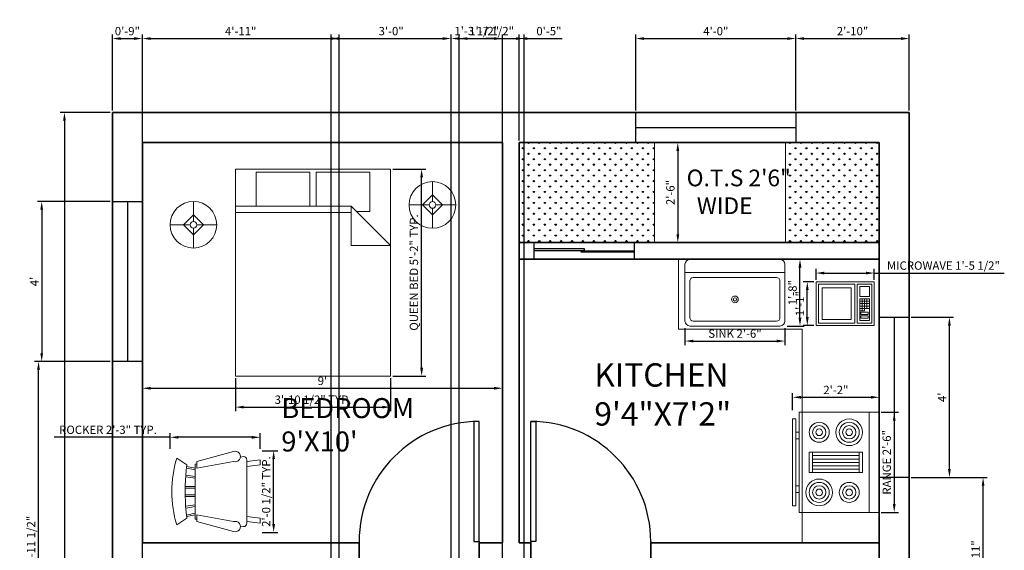
# Model space of a CAD drawing. Units: inches. Extents: x 2459 to 2755, y 1300 to 1776.
# Tile 4 of 4: x 2459 to 2755, y 1617 to 1776. Entities that reach past the tile are written whole.
import ezdxf

# ---------------------------------------------------------------- set-up
doc = ezdxf.new("R2010")
doc.units = ezdxf.units.IN
for name, color, linetype, lineweight in [('A-AREA-IDEN', 3, 'Continuous', 25), ('A-EQPM', 9, 'Continuous', 18), ('A-FLOR-CASE', 7, 'Continuous', 20), ('A-FLOR-FIXT', 8, 'Continuous', 18), ('A-WALL', 7, 'Continuous', 35), ('DIM', 4, 'Continuous', 18), ('DOOR', 20, 'Continuous', 25), ('FURNITURE', 6, 'Continuous', 18), ('L-PLNT', 3, 'Continuous', 18), ('L-PLNT-PATT', 8, 'Continuous', 13), ('WIN', 2, 'Continuous', 25)]:
    doc.layers.add(name, color=color, linetype=linetype, lineweight=lineweight)
doc.styles.get("Standard").update_dxf_attribs({"font": 'arial.ttf'})
doc.dimstyles.new('ISO-25', dxfattribs={"dimtxt": 2.5, "dimasz": 2.5, "dimexe": 1.25, "dimexo": 0.625, "dimtad": 1, "dimlunit": 3, "dimtxsty": 'Standard', "dimcen": 2.5, "dimadec": 0, "dimazin": 0, "dimtfac": 1, "dimtmove": 0, "dimatfit": 3, "dimfxl": 1, "dimarcsym": 0})

# ---------------------------------------------------------------- blocks, each defined once
blk = doc.blocks.new('*U2')
for p, q in [((0, 0), (0, -6)), ((40, 0), (40, -6))]:
    blk.add_line(p, q)
blk.add_lwpolyline([(0, 0), (0, 40), (1.75, 40), (1.75, 0)], close=True)
blk.add_arc((0, 0), 40, 0, 90)
blk = doc.blocks.new('*U3')
for p, q in [((0, 0), (0, -6)), ((-40, 0), (-40, -6))]:
    blk.add_line(p, q)
blk.add_lwpolyline([(0, 0), (0, 40), (-1.75, 40), (-1.75, 0)], close=True)
blk.add_arc((0, 0), 40, 90, 180)
blk = doc.blocks.new('Bed - Queen')
for p, q in [((0, -80.00003), (0, 0)), ((0, 0), (59.99999, 0)), ((59.99999, 0), (59.99999, -80.00003)), ((7.99999, -1.2), (28.79998, -1.2)), ((7.99999, -14.4), (7.99999, -1.2)), ((28.79998, -1.2), (28.79998, -14.4)), ((31.19999, -1.2), (51.99999, -1.2)), ((31.19999, -14.4), (31.19999, -1.2)), ((51.99999, -1.2), (51.99999, -16.4)), ((0, -14.4), (44.8, -14.4)), ((59.99999, -29.6), (44.8, -14.4)), ((44.8, -14.4), (44.8, -29.6)), ((44.8, -16.8), (0, -16.8)), ((51.99999, -16.4), (46.79936, -16.4)), ((44.8, -29.6), (59.99999, -29.6)), ((59.99999, -80.00003), (0, -80.00003))]:
    blk.add_line(p, q)
blk = doc.blocks.new('Microwave')
for p, q in [((18, 10), (22, 10)), ((22, 9), (18, 9)), ((19, 7), (19, 11)), ((20, 11), (20, 7)), ((21, 7), (21, 11)), ((18, 8), (22, 8)), ((22, 7), (18, 7)), ((20, 6), (18, 6)), ((19, 6), (19, 7)), ((20, 7), (20, 6))]:
    blk.add_line(p, q)
for points in [[(0, 0), (0, 18), (24, 18), (24, 0)], [(1, 1), (1, 17), (16, 17), (16, 1)], [(17, 1), (17, 17), (23, 17), (23, 1)], [(2.5, 2.5), (2.5, 15.5), (14.5, 15.5), (14.5, 2.5)], [(18, 12), (18, 16), (22, 16), (22, 12)], [(18, 2), (18, 11), (22, 11), (22, 2)], [(18.5, 4.5), (18.5, 5.5), (21.5, 5.5), (21.5, 4.5)], [(18.5, 3), (18.5, 4), (21.5, 4), (21.5, 3)]]:
    blk.add_lwpolyline(points, close=True)
blk = doc.blocks.new('Range-Oven - 30 in top')
for p, q in [((0, -3), (30, -3)), ((12, -6), (18, -6)), ((13, -20), (13, -6)), ((14, -6), (14, -20)), ((15, -20), (15, -6)), ((16, -6), (16, -20)), ((17, -20), (17, -6)), ((18, -20), (12, -20)), ((6, -24), (6, -25)), ((8, -25), (8, -24)), ((22, -25), (22, -24)), ((24, -24), (24, -25))]:
    blk.add_line(p, q)
for points in [[(0, -24), (0, 0), (30, 0), (30, -24)], [(12, -21), (12, -5), (18, -5), (18, -21)], [(2, -26), (2, -25), (28, -25), (28, -26)]]:
    blk.add_lwpolyline(points, close=True)
for centre, radius in [((6, -9), 4), ((6, -9), 3), ((6, -9), 2), ((6, -9), 1), ((24, -9), 3), ((24, -9), 2), ((24, -9), 1), ((24, -18), 4), ((6, -18), 3), ((6, -18), 2), ((6, -18), 1), ((24, -18), 3), ((24, -18), 2), ((24, -18), 1)]:
    blk.add_circle(centre, radius)
blk = doc.blocks.new('Sink-single - 30 in top')
blk.add_line((-15, -3.999996), (15, -3.999996))
for points in [[(-13.5, 0), (13.5, 0)], [(-15, -18.499996), (-15, -1.5)], [(15, -1.5), (15, -18.499996)], [(-12.5, -5.499996), (12.5, -5.499996)], [(-13.5, -17.499996), (-13.5, -6.499996)], [(13.5, -6.499996), (13.5, -17.499996)], [(13.5, -19.999996), (-13.5, -19.999996)], [(12.5, -18.499996), (-12.5, -18.499996)]]:
    blk.add_lwpolyline(points)
for radius in [1, 0.5]:
    blk.add_circle((0, -11.999996), radius)
for centre, radius, start, end in [((-13.5, -1.5), 1.5, 90, 180), ((13.5, -1.5), 1.5, 0, 90), ((-12.5, -6.499996), 1, 90, 180), ((12.5, -6.499996), 1, 0, 90), ((-12.5, -17.499996), 1, 180, 270), ((12.5, -17.499996), 1, 270, 0), ((-13.5, -18.499996), 1.5, 180, 270), ((13.5, -18.499996), 1.5, 270, 0)]:
    blk.add_arc(centre, radius, start, end)
blk = doc.blocks.new('Lamp - Table')
for p, q in [((0, 7), (0, 1)), ((0, 3), (-3, 0)), ((3, 0), (0, 3)), ((-1, 0), (-7, 0)), ((-3, 0), (0, -3)), ((0, -3), (3, 0)), ((1, 0), (7, 0)), ((0, -1), (0, -7))]:
    blk.add_line(p, q)
for radius in [7, 1]:
    blk.add_circle((0, 0), radius)
blk = doc.blocks.new('Chair - Rocking')
for p, q in [((-8, -4.5), (-10, -1.5)), ((8, -4.5), (10, -1.5)), ((-7.5, -4.5), (-7, -7)), ((-6.5, -7), (-7.02225, -4.43)), ((-4.5, -7), (-4.96674, -4.19951)), ((-4, -7), (-4.40532, -4.16272)), ((-1.5, -4.05012), (-1.5, -7)), ((-1, -7), (-1, -4.05012)), ((1, -7), (1, -4.04655)), ((1.5, -4.05012), (1.5, -7)), ((4, -7), (4.40187, -4.18694)), ((4.5, -7), (4.96761, -4.19437)), ((6.5, -7), (7, -4.4057)), ((7.5, -4.5), (7, -7)), ((-9, -7.5), (-12, -18.49999)), ((-7, -7.5), (-9, -7.5)), ((-9, -18.49999), (-7, -7.5)), ((-8.23428, -6.99939), (-8.3093, -7.47958)), ((-8.23041, -7), (8.23915, -7)), ((7, -7.5), (9, -7.5)), ((9, -18.49999), (7, -7.5)), ((8.31071, -7.48854), (8.23449, -7.00073)), ((9, -7.5), (12, -18.49999)), ((-10.36644, -20.64523), (-10.5, -21.49999)), ((10.5, -21.49999), (10.3575, -20.58798)), ((-9, -22.49999), (-9.5, -26.49999)), ((0, -22.49999), (-9.5, -22.49999)), ((-8, -26.49999), (-7.5, -22.49999)), ((0, -22.49999), (9.5, -22.49999)), ((8, -26.49999), (7.5, -22.49999)), ((9, -22.49999), (9.5, -26.49999)), ((-9.5, -26.49999), (-8, -26.49999)), ((9.5, -26.49999), (8, -26.49999))]:
    blk.add_line(p, q)
for centre, radius, start, end in [((0, -34.08333), 34.08333, 72.93847, 107.0615), ((0, -68.25004), 64.25, 93.92211, 97.15267), ((0, -68.25004), 64.25, 82.84733, 93.92211), ((-10.5, -18.99999), 1.58114, 161.5651, 18.43495), ((10.5, -18.99999), 1.58114, 161.5651, 18.43495), ((-9.5, -21.49999), 1, 180, 270), ((9.5, -21.49999), 1, 270, 0)]:
    blk.add_arc(centre, radius, start, end)
blk = doc.blocks.new('*D19')
at = {"layer": 'Defpoints', "color": 0, "transparency": 16777216}
for p in [(2487, 1748.32), (2472.62, 1324.32), (2487, 1324.32)]:
    blk.add_point(p, dxfattribs=at)
at = {"layer": 'DIM', "color": 0, "lineweight": -2, "transparency": 16777216}
for p, q in [((2486.37, 1748.32), (2471.37, 1748.32)), ((2472.62, 1745.82), (2472.62, 1326.82)), ((2486.37, 1324.32), (2471.37, 1324.32))]:
    blk.add_line(p, q, dxfattribs=at)
at = {"layer": 'DIM', "color": 0, "transparency": 16777216}
for points in [[(2472.2, 1745.82), (2473.04, 1745.82), (2472.62, 1748.32)], [(2472.2, 1326.82), (2473.04, 1326.82), (2472.62, 1324.32)]]:
    blk.add_solid(points, dxfattribs=at)
at = {"layer": 'DIM', "color": 0, "transparency": 16777216, "insert": (2470.72, 1536.32), "char_height": 2.5, "attachment_point": 5, "rotation": 90}
blk.add_mtext('35\'-4"', dxfattribs=at)
blk = doc.blocks.new('*D20')
at = {"layer": 'Defpoints', "color": 0, "transparency": 16777216}
for p in [(2487, 1721.67), (2465.8, 1673.67), (2487, 1673.67)]:
    blk.add_point(p, dxfattribs=at)
at = {"layer": 'DIM', "color": 0, "lineweight": -2, "transparency": 16777216}
for p, q in [((2486.37, 1721.67), (2464.55, 1721.67)), ((2465.8, 1719.17), (2465.8, 1676.17)), ((2486.37, 1673.67), (2464.55, 1673.67))]:
    blk.add_line(p, q, dxfattribs=at)
at = {"layer": 'DIM', "color": 0, "transparency": 16777216}
for points in [[(2465.38, 1719.17), (2466.22, 1719.17), (2465.8, 1721.67)], [(2465.38, 1676.17), (2466.22, 1676.17), (2465.8, 1673.67)]]:
    blk.add_solid(points, dxfattribs=at)
at = {"layer": 'DIM', "color": 0, "transparency": 16777216, "insert": (2463.93, 1697.67), "char_height": 2.5, "attachment_point": 5, "rotation": 90}
blk.add_mtext("4'", dxfattribs=at)
blk = doc.blocks.new('*D29')
at = {"layer": 'Defpoints', "color": 0, "transparency": 16777216}
for p in [(2726, 1686.95), (2738.05, 1686.95), (2726, 1638.95)]:
    blk.add_point(p, dxfattribs=at)
at = {"layer": 'DIM', "color": 0, "lineweight": -2, "transparency": 16777216}
for p, q in [((2726.62, 1686.95), (2739.3, 1686.95)), ((2738.05, 1641.45), (2738.05, 1684.45)), ((2726.62, 1638.95), (2739.3, 1638.95))]:
    blk.add_line(p, q, dxfattribs=at)
at = {"layer": 'DIM', "color": 0, "transparency": 16777216}
for points in [[(2737.63, 1684.45), (2738.46, 1684.45), (2738.05, 1686.95)], [(2737.63, 1641.45), (2738.46, 1641.45), (2738.05, 1638.95)]]:
    blk.add_solid(points, dxfattribs=at)
at = {"layer": 'DIM', "color": 0, "transparency": 16777216, "insert": (2736.17, 1662.95), "char_height": 2.5, "attachment_point": 5, "rotation": 90}
blk.add_mtext("4'", dxfattribs=at)
blk = doc.blocks.new('*D30')
at = {"layer": 'Defpoints', "color": 0, "transparency": 16777216}
for p in [(2649.55, 1739.32), (2649.55, 1709.32), (2656.59, 1709.32)]:
    blk.add_point(p, dxfattribs=at)
at = {"layer": 'DIM', "color": 0, "lineweight": -2, "transparency": 16777216}
for p, q in [((2650.18, 1739.32), (2657.84, 1739.32)), ((2656.59, 1736.82), (2656.59, 1711.82)), ((2650.18, 1709.32), (2657.84, 1709.32))]:
    blk.add_line(p, q, dxfattribs=at)
at = {"layer": 'DIM', "color": 0, "transparency": 16777216}
for points in [[(2656.17, 1736.82), (2657.01, 1736.82), (2656.59, 1739.32)], [(2656.17, 1711.82), (2657.01, 1711.82), (2656.59, 1709.32)]]:
    blk.add_solid(points, dxfattribs=at)
at = {"layer": 'DIM', "color": 0, "transparency": 16777216, "insert": (2654.69, 1724.32), "char_height": 2.5, "attachment_point": 5, "rotation": 90}
blk.add_mtext('2\'-6"', dxfattribs=at)
blk = doc.blocks.new('*D33')
at = {"layer": 'Defpoints', "color": 0, "transparency": 16777216}
for p in [(2496, 1665.67), (2604, 1665.67), (2604, 1665.67)]:
    blk.add_point(p, dxfattribs=at)
at = {"layer": 'DIM', "color": 0, "lineweight": -2, "transparency": 16777216}
for p, q in [((2496, 1666.29), (2496, 1666.92)), ((2498.5, 1665.67), (2601.5, 1665.67)), ((2604, 1666.29), (2604, 1666.92))]:
    blk.add_line(p, q, dxfattribs=at)
at = {"layer": 'DIM', "color": 0, "transparency": 16777216}
for points in [[(2498.5, 1666.09), (2498.5, 1665.25), (2496, 1665.67)], [(2601.5, 1666.09), (2601.5, 1665.25), (2604, 1665.67)]]:
    blk.add_solid(points, dxfattribs=at)
at = {"layer": 'DIM', "color": 0, "transparency": 16777216, "insert": (2550, 1667.57), "char_height": 2.5, "attachment_point": 5}
blk.add_mtext("9'", dxfattribs=at)
blk = doc.blocks.new('WIN-48IN')
blk.add_line((4.5, 48), (4.5, 0))
blk.add_lwpolyline([(0, 48), (9, 48), (9, 0), (0, 0)], close=True)
blk = doc.blocks.new('*D37')
at = {"layer": 'Defpoints', "color": 0, "transparency": 16777216}
for p in [(2570.45, 1731.37), (2579.75, 1731.37), (2570.45, 1669.32)]:
    blk.add_point(p, dxfattribs=at)
at = {"layer": 'DIM', "color": 0, "lineweight": -2, "transparency": 16777216}
for p, q in [((2571.07, 1731.37), (2581, 1731.37)), ((2579.75, 1671.82), (2579.75, 1728.87)), ((2571.07, 1669.32), (2581, 1669.32))]:
    blk.add_line(p, q, dxfattribs=at)
at = {"layer": 'DIM', "color": 0, "transparency": 16777216}
for points in [[(2579.34, 1728.87), (2580.17, 1728.87), (2579.75, 1731.37)], [(2579.34, 1671.82), (2580.17, 1671.82), (2579.75, 1669.32)]]:
    blk.add_solid(points, dxfattribs=at)
at = {"layer": 'DIM', "color": 0, "transparency": 16777216, "insert": (2577.76, 1700.35), "char_height": 2.5, "attachment_point": 5, "rotation": 90}
blk.add_mtext('QUEEN BED 5\'-2" TYP.', dxfattribs=at)
blk = doc.blocks.new('*D38')
at = {"layer": 'Defpoints', "color": 0, "transparency": 16777216}
for p in [(2523.91, 1669.32), (2570.45, 1669.32), (2570.45, 1660.02)]:
    blk.add_point(p, dxfattribs=at)
at = {"layer": 'DIM', "color": 0, "lineweight": -2, "transparency": 16777216}
for p, q in [((2523.91, 1668.7), (2523.91, 1658.77)), ((2570.45, 1668.7), (2570.45, 1658.77)), ((2526.41, 1660.02), (2567.95, 1660.02))]:
    blk.add_line(p, q, dxfattribs=at)
at = {"layer": 'DIM', "color": 0, "transparency": 16777216}
for points in [[(2526.41, 1660.43), (2526.41, 1659.6), (2523.91, 1660.02)], [(2567.95, 1660.43), (2567.95, 1659.6), (2570.45, 1660.02)]]:
    blk.add_solid(points, dxfattribs=at)
at = {"layer": 'DIM', "color": 0, "transparency": 16777216, "insert": (2547.18, 1661.93), "char_height": 2.5, "attachment_point": 5}
blk.add_mtext('3\'-10 1/2" TYP.', dxfattribs=at)
blk = doc.blocks.new('*D41')
at = {"layer": 'Defpoints', "color": 0, "transparency": 16777216}
for p in [(2504.32, 1650.98), (2504.32, 1646.93), (2531.32, 1646.93)]:
    blk.add_point(p, dxfattribs=at)
at = {"layer": 'DIM', "color": 0, "lineweight": -2, "transparency": 16777216}
for p, q in [((2504.32, 1650.98), (2469.55, 1650.98)), ((2504.32, 1647.55), (2504.32, 1652.23)), ((2528.82, 1650.98), (2506.82, 1650.98)), ((2531.32, 1647.55), (2531.32, 1652.23))]:
    blk.add_line(p, q, dxfattribs=at)
at = {"layer": 'DIM', "color": 0, "transparency": 16777216}
for points in [[(2506.82, 1651.39), (2506.82, 1650.56), (2504.32, 1650.98)], [(2528.82, 1651.39), (2528.82, 1650.56), (2531.32, 1650.98)]]:
    blk.add_solid(points, dxfattribs=at)
at = {"layer": 'DIM', "color": 0, "transparency": 16777216, "insert": (2485.68, 1652.9), "char_height": 2.5, "attachment_point": 5}
blk.add_mtext('ROCKER 2\'-3" TYP.', dxfattribs=at)
blk = doc.blocks.new('*D42')
at = {"layer": 'Defpoints', "color": 0, "transparency": 16777216}
for p in [(2531.32, 1646.93), (2535.37, 1646.93), (2531.32, 1622.49)]:
    blk.add_point(p, dxfattribs=at)
at = {"layer": 'DIM', "color": 0, "lineweight": -2, "transparency": 16777216}
for p, q in [((2531.94, 1646.93), (2536.62, 1646.93)), ((2535.37, 1624.99), (2535.37, 1644.43)), ((2531.94, 1622.49), (2536.62, 1622.49))]:
    blk.add_line(p, q, dxfattribs=at)
at = {"layer": 'DIM', "color": 0, "transparency": 16777216}
for points in [[(2534.95, 1644.43), (2535.79, 1644.43), (2535.37, 1646.93)], [(2534.95, 1624.99), (2535.79, 1624.99), (2535.37, 1622.49)]]:
    blk.add_solid(points, dxfattribs=at)
at = {"layer": 'DIM', "color": 0, "transparency": 16777216, "insert": (2533.45, 1634.71), "char_height": 2.5, "attachment_point": 5, "rotation": 90}
blk.add_mtext('2\'-0 1/2" TYP.', dxfattribs=at)
blk = doc.blocks.new('*D49')
at = {"layer": 'Defpoints', "color": 0, "transparency": 16777216}
for p in [(2715.51, 1700.19), (2698.05, 1697.57), (2715.51, 1697.57)]:
    blk.add_point(p, dxfattribs=at)
at = {"layer": 'DIM', "color": 0, "lineweight": -2, "transparency": 16777216}
for p, q in [((2698.05, 1698.2), (2698.05, 1701.44)), ((2715.51, 1698.2), (2715.51, 1701.44)), ((2700.55, 1700.19), (2713.01, 1700.19)), ((2715.51, 1700.19), (2754.51, 1700.19))]:
    blk.add_line(p, q, dxfattribs=at)
at = {"layer": 'DIM', "color": 0, "transparency": 16777216}
for points in [[(2700.55, 1700.61), (2700.55, 1699.78), (2698.05, 1700.19)], [(2713.01, 1700.61), (2713.01, 1699.78), (2715.51, 1700.19)]]:
    blk.add_solid(points, dxfattribs=at)
at = {"layer": 'DIM', "color": 0, "transparency": 16777216, "insert": (2736.26, 1702.11), "char_height": 2.5, "attachment_point": 5}
blk.add_mtext('MICROWAVE 1\'-5 1/2"', dxfattribs=at)
blk = doc.blocks.new('*D50')
at = {"layer": 'Defpoints', "color": 0, "transparency": 16777216}
for p in [(2695.43, 1697.57), (2698.05, 1697.57), (2698.05, 1684.48)]:
    blk.add_point(p, dxfattribs=at)
at = {"layer": 'DIM', "color": 0, "lineweight": -2, "transparency": 16777216}
for p, q in [((2697.42, 1697.57), (2694.18, 1697.57)), ((2695.43, 1686.98), (2695.43, 1695.07)), ((2697.42, 1684.48), (2694.18, 1684.48))]:
    blk.add_line(p, q, dxfattribs=at)
at = {"layer": 'DIM', "color": 0, "transparency": 16777216}
for points in [[(2695.01, 1695.07), (2695.84, 1695.07), (2695.43, 1697.57)], [(2695.01, 1686.98), (2695.84, 1686.98), (2695.43, 1684.48)]]:
    blk.add_solid(points, dxfattribs=at)
at = {"layer": 'DIM', "color": 0, "transparency": 16777216, "insert": (2693.55, 1691.02), "char_height": 2.5, "attachment_point": 5, "rotation": 90}
blk.add_mtext('1\'-1"', dxfattribs=at)
blk = doc.blocks.new('*D51')
at = {"layer": 'Defpoints', "color": 0, "transparency": 16777216}
for p in [(2717, 1658.47), (2717, 1628.47), (2721.5, 1628.47)]:
    blk.add_point(p, dxfattribs=at)
at = {"layer": 'DIM', "color": 0, "lineweight": -2, "transparency": 16777216}
for p, q in [((2717.62, 1658.47), (2722.75, 1658.47)), ((2721.5, 1655.97), (2721.5, 1630.97)), ((2717.62, 1628.47), (2722.75, 1628.47))]:
    blk.add_line(p, q, dxfattribs=at)
at = {"layer": 'DIM', "color": 0, "transparency": 16777216}
for points in [[(2721.08, 1655.97), (2721.91, 1655.97), (2721.5, 1658.47)], [(2721.08, 1630.97), (2721.91, 1630.97), (2721.5, 1628.47)]]:
    blk.add_solid(points, dxfattribs=at)
at = {"layer": 'DIM', "color": 0, "transparency": 16777216, "insert": (2719.58, 1643.47), "char_height": 2.5, "attachment_point": 5, "rotation": 90}
blk.add_mtext('RANGE 2\'-6"', dxfattribs=at)
blk = doc.blocks.new('*D52')
at = {"layer": 'Defpoints', "color": 0, "transparency": 16777216}
for p in [(2717, 1662.97), (2691, 1658.47), (2717, 1658.47)]:
    blk.add_point(p, dxfattribs=at)
at = {"layer": 'DIM', "color": 0, "lineweight": -2, "transparency": 16777216}
for p, q in [((2691, 1659.1), (2691, 1664.22)), ((2693.5, 1662.97), (2714.5, 1662.97)), ((2717, 1659.1), (2717, 1664.22))]:
    blk.add_line(p, q, dxfattribs=at)
at = {"layer": 'DIM', "color": 0, "transparency": 16777216}
for points in [[(2693.5, 1663.39), (2693.5, 1662.56), (2691, 1662.97)], [(2714.5, 1663.39), (2714.5, 1662.56), (2717, 1662.97)]]:
    blk.add_solid(points, dxfattribs=at)
at = {"layer": 'DIM', "color": 0, "transparency": 16777216, "insert": (2704, 1664.85), "char_height": 2.5, "attachment_point": 5}
blk.add_mtext('2\'-2"', dxfattribs=at)
blk = doc.blocks.new('*D53')
at = {"layer": 'Defpoints', "color": 0, "transparency": 16777216}
for p in [(2658.73, 1684.32), (2688.73, 1684.32), (2688.73, 1679.82)]:
    blk.add_point(p, dxfattribs=at)
at = {"layer": 'DIM', "color": 0, "lineweight": -2, "transparency": 16777216}
for p, q in [((2658.73, 1683.69), (2658.73, 1678.57)), ((2688.73, 1683.69), (2688.73, 1678.57)), ((2661.23, 1679.82), (2686.23, 1679.82))]:
    blk.add_line(p, q, dxfattribs=at)
at = {"layer": 'DIM', "color": 0, "transparency": 16777216}
for points in [[(2661.23, 1680.23), (2661.23, 1679.4), (2658.73, 1679.82)], [(2686.23, 1680.23), (2686.23, 1679.4), (2688.73, 1679.82)]]:
    blk.add_solid(points, dxfattribs=at)
at = {"layer": 'DIM', "color": 0, "transparency": 16777216, "insert": (2673.73, 1681.73), "char_height": 2.5, "attachment_point": 5}
blk.add_mtext('SINK 2\'-6"', dxfattribs=at)
blk = doc.blocks.new('*D54')
at = {"layer": 'Defpoints', "color": 0, "transparency": 16777216}
for p in [(2688.73, 1704.32), (2693.23, 1704.32), (2688.73, 1684.32)]:
    blk.add_point(p, dxfattribs=at)
at = {"layer": 'DIM', "color": 0, "lineweight": -2, "transparency": 16777216}
for p, q in [((2689.36, 1704.32), (2694.48, 1704.32)), ((2693.23, 1686.82), (2693.23, 1701.82)), ((2689.36, 1684.32), (2694.48, 1684.32))]:
    blk.add_line(p, q, dxfattribs=at)
at = {"layer": 'DIM', "color": 0, "transparency": 16777216}
for points in [[(2692.81, 1701.82), (2693.65, 1701.82), (2693.23, 1704.32)], [(2692.81, 1686.82), (2693.65, 1686.82), (2693.23, 1684.32)]]:
    blk.add_solid(points, dxfattribs=at)
at = {"layer": 'DIM', "color": 0, "transparency": 16777216, "insert": (2691.33, 1694.32), "char_height": 2.5, "attachment_point": 5, "rotation": 90}
blk.add_mtext('1\'-8"', dxfattribs=at)
blk = doc.blocks.new('*D58')
at = {"layer": 'Defpoints', "color": 0, "transparency": 16777216}
for p in [(2496, 1770.47), (2487, 1748.32), (2496, 1739.32)]:
    blk.add_point(p, dxfattribs=at)
at = {"layer": 'DIM', "color": 0, "lineweight": -2, "transparency": 16777216}
for p, q in [((2487, 1748.94), (2487, 1771.72)), ((2489.5, 1770.47), (2493.5, 1770.47)), ((2496, 1739.94), (2496, 1771.72))]:
    blk.add_line(p, q, dxfattribs=at)
at = {"layer": 'DIM', "color": 0, "transparency": 16777216}
for points in [[(2489.5, 1770.88), (2489.5, 1770.05), (2487, 1770.47)], [(2493.5, 1770.88), (2493.5, 1770.05), (2496, 1770.47)]]:
    blk.add_solid(points, dxfattribs=at)
at = {"layer": 'DIM', "color": 0, "transparency": 16777216, "insert": (2491.5, 1772.37), "char_height": 2.5, "attachment_point": 5}
blk.add_mtext('0\'-9"', dxfattribs=at)
blk = doc.blocks.new('*D59')
at = {"layer": 'Defpoints', "color": 0, "transparency": 16777216}
for p in [(2609, 1770.47), (2604, 1739.32), (2609, 1739.32)]:
    blk.add_point(p, dxfattribs=at)
at = {"layer": 'DIM', "color": 0, "lineweight": -2, "transparency": 16777216}
for p, q in [((2601.5, 1770.47), (2599, 1770.47)), ((2604, 1739.94), (2604, 1771.72)), ((2604, 1770.47), (2609, 1770.47)), ((2609, 1739.94), (2609, 1771.72)), ((2611.5, 1770.47), (2621.89, 1770.47))]:
    blk.add_line(p, q, dxfattribs=at)
at = {"layer": 'DIM', "color": 0, "transparency": 16777216}
for points in [[(2601.5, 1770.88), (2601.5, 1770.05), (2604, 1770.47)], [(2611.5, 1770.88), (2611.5, 1770.05), (2609, 1770.47)]]:
    blk.add_solid(points, dxfattribs=at)
at = {"layer": 'DIM', "color": 0, "transparency": 16777216, "insert": (2617.94, 1772.37), "char_height": 2.5, "attachment_point": 5}
blk.add_mtext('0\'-5"', dxfattribs=at)
blk = doc.blocks.new('*D60')
at = {"layer": 'Defpoints', "color": 0, "transparency": 16777216}
for p in [(2691.98, 1770.47), (2643.98, 1748.32), (2691.98, 1748.32)]:
    blk.add_point(p, dxfattribs=at)
at = {"layer": 'DIM', "color": 0, "lineweight": -2, "transparency": 16777216}
for p, q in [((2643.98, 1748.94), (2643.98, 1771.72)), ((2646.48, 1770.47), (2689.48, 1770.47)), ((2691.98, 1748.94), (2691.98, 1771.72))]:
    blk.add_line(p, q, dxfattribs=at)
at = {"layer": 'DIM', "color": 0, "transparency": 16777216}
for points in [[(2646.48, 1770.88), (2646.48, 1770.05), (2643.98, 1770.47)], [(2689.48, 1770.88), (2689.48, 1770.05), (2691.98, 1770.47)]]:
    blk.add_solid(points, dxfattribs=at)
at = {"layer": 'DIM', "color": 0, "transparency": 16777216, "insert": (2667.98, 1772.37), "char_height": 2.5, "attachment_point": 5}
blk.add_mtext('4\'-0"', dxfattribs=at)
blk = doc.blocks.new('*D61')
at = {"layer": 'Defpoints', "color": 0, "transparency": 16777216}
for p in [(2726, 1770.47), (2691.98, 1748.32), (2726, 1748.32)]:
    blk.add_point(p, dxfattribs=at)
at = {"layer": 'DIM', "color": 0, "lineweight": -2, "transparency": 16777216}
for p, q in [((2691.98, 1748.94), (2691.98, 1771.72)), ((2694.48, 1770.47), (2723.5, 1770.47)), ((2726, 1748.94), (2726, 1771.72))]:
    blk.add_line(p, q, dxfattribs=at)
at = {"layer": 'DIM', "color": 0, "transparency": 16777216}
for points in [[(2694.48, 1770.88), (2694.48, 1770.05), (2691.98, 1770.47)], [(2723.5, 1770.88), (2723.5, 1770.05), (2726, 1770.47)]]:
    blk.add_solid(points, dxfattribs=at)
at = {"layer": 'DIM', "color": 0, "transparency": 16777216, "insert": (2708.99, 1772.37), "char_height": 2.5, "attachment_point": 5}
blk.add_mtext('2\'-10"', dxfattribs=at)
blk = doc.blocks.new('*D64')
at = {"layer": 'Defpoints', "color": 0, "transparency": 16777216}
for p in [(2464.85, 1673.67), (2487, 1673.67), (2487, 1565.93)]:
    blk.add_point(p, dxfattribs=at)
at = {"layer": 'DIM', "color": 0, "lineweight": -2, "transparency": 16777216}
for p, q in [((2486.37, 1673.67), (2463.6, 1673.67)), ((2464.85, 1568.43), (2464.85, 1671.17)), ((2486.37, 1565.93), (2463.6, 1565.93))]:
    blk.add_line(p, q, dxfattribs=at)
at = {"layer": 'DIM', "color": 0, "transparency": 16777216}
for points in [[(2464.43, 1671.17), (2465.26, 1671.17), (2464.85, 1673.67)], [(2464.43, 1568.43), (2465.26, 1568.43), (2464.85, 1565.93)]]:
    blk.add_solid(points, dxfattribs=at)
at = {"layer": 'DIM', "color": 0, "transparency": 16777216, "insert": (2462.93, 1619.8), "char_height": 2.5, "attachment_point": 5, "rotation": 90}
blk.add_mtext('8\'-11 1/2"', dxfattribs=at)
blk = doc.blocks.new('*D69')
at = {"layer": 'Defpoints', "color": 0, "transparency": 16777216}
for p in [(2726, 1638.95), (2748.15, 1638.95), (2726, 1591.84)]:
    blk.add_point(p, dxfattribs=at)
at = {"layer": 'DIM', "color": 0, "lineweight": -2, "transparency": 16777216}
for p, q in [((2726.62, 1638.95), (2749.4, 1638.95)), ((2748.15, 1594.34), (2748.15, 1636.45)), ((2726.62, 1591.84), (2749.4, 1591.84))]:
    blk.add_line(p, q, dxfattribs=at)
at = {"layer": 'DIM', "color": 0, "transparency": 16777216}
for points in [[(2747.73, 1636.45), (2748.56, 1636.45), (2748.15, 1638.95)], [(2747.73, 1594.34), (2748.56, 1594.34), (2748.15, 1591.84)]]:
    blk.add_solid(points, dxfattribs=at)
at = {"layer": 'DIM', "color": 0, "transparency": 16777216, "insert": (2746.24, 1615.39), "char_height": 2.5, "attachment_point": 5, "rotation": 90}
blk.add_mtext('3\'-11"', dxfattribs=at)
blk = doc.blocks.new('*D70')
at = {"layer": 'Defpoints', "color": 0, "transparency": 16777216}
for p in [(2588.61, 1770.47), (2552.61, 1374.32), (2588.61, 1374.32)]:
    blk.add_point(p, dxfattribs=at)
at = {"layer": 'DIM', "color": 0, "lineweight": -2, "transparency": 16777216}
for p, q in [((2552.61, 1374.94), (2552.61, 1771.72)), ((2555.11, 1770.47), (2586.11, 1770.47)), ((2588.61, 1374.94), (2588.61, 1771.72))]:
    blk.add_line(p, q, dxfattribs=at)
at = {"layer": 'DIM', "color": 0, "transparency": 16777216}
for points in [[(2555.11, 1770.88), (2555.11, 1770.05), (2552.61, 1770.47)], [(2586.11, 1770.88), (2586.11, 1770.05), (2588.61, 1770.47)]]:
    blk.add_solid(points, dxfattribs=at)
at = {"layer": 'DIM', "color": 0, "transparency": 16777216, "insert": (2570.61, 1772.37), "char_height": 2.5, "attachment_point": 5}
blk.add_mtext('3\'-0"', dxfattribs=at)
blk = doc.blocks.new('*D77')
at = {"layer": 'Defpoints', "color": 0, "transparency": 16777216}
for p in [(2554.97, 1770.47), (2496, 1458.32), (2554.97, 1458.32)]:
    blk.add_point(p, dxfattribs=at)
at = {"layer": 'DIM', "color": 0, "lineweight": -2, "transparency": 16777216}
for p, q in [((2496, 1458.94), (2496, 1771.72)), ((2498.5, 1770.47), (2552.47, 1770.47)), ((2554.97, 1458.94), (2554.97, 1771.72))]:
    blk.add_line(p, q, dxfattribs=at)
at = {"layer": 'DIM', "color": 0, "transparency": 16777216}
for points in [[(2498.5, 1770.88), (2498.5, 1770.05), (2496, 1770.47)], [(2552.47, 1770.88), (2552.47, 1770.05), (2554.97, 1770.47)]]:
    blk.add_solid(points, dxfattribs=at)
at = {"layer": 'DIM', "color": 0, "transparency": 16777216, "insert": (2525.48, 1772.35), "char_height": 2.5, "attachment_point": 5}
blk.add_mtext('4\'-11"', dxfattribs=at)
blk = doc.blocks.new('*D78')
at = {"layer": 'Defpoints', "color": 0, "transparency": 16777216}
for p in [(2610.51, 1770.47), (2590.97, 1458.32), (2610.51, 1458.32)]:
    blk.add_point(p, dxfattribs=at)
at = {"layer": 'DIM', "color": 0, "lineweight": -2, "transparency": 16777216}
for p, q in [((2590.97, 1458.94), (2590.97, 1771.72)), ((2593.47, 1770.47), (2608.01, 1770.47)), ((2610.51, 1458.94), (2610.51, 1771.72))]:
    blk.add_line(p, q, dxfattribs=at)
at = {"layer": 'DIM', "color": 0, "transparency": 16777216}
for points in [[(2593.47, 1770.88), (2593.47, 1770.05), (2590.97, 1770.47)], [(2608.01, 1770.88), (2608.01, 1770.05), (2610.51, 1770.47)]]:
    blk.add_solid(points, dxfattribs=at)
at = {"layer": 'DIM', "color": 0, "transparency": 16777216, "insert": (2600.74, 1772.38), "char_height": 2.5, "attachment_point": 5}
blk.add_mtext('1\'-7 1/2"', dxfattribs=at)
blk = doc.blocks.new('*D79')
at = {"layer": 'Defpoints', "color": 0, "transparency": 16777216}
for p in [(2604, 1770.47), (2588.61, 1374.32), (2604, 1374.32)]:
    blk.add_point(p, dxfattribs=at)
at = {"layer": 'DIM', "color": 0, "lineweight": -2, "transparency": 16777216}
for p, q in [((2588.61, 1374.94), (2588.61, 1771.72)), ((2591.11, 1770.47), (2601.5, 1770.47)), ((2604, 1374.94), (2604, 1771.72))]:
    blk.add_line(p, q, dxfattribs=at)
at = {"layer": 'DIM', "color": 0, "transparency": 16777216}
for points in [[(2591.11, 1770.88), (2591.11, 1770.05), (2588.61, 1770.47)], [(2601.5, 1770.88), (2601.5, 1770.05), (2604, 1770.47)]]:
    blk.add_solid(points, dxfattribs=at)
at = {"layer": 'DIM', "color": 0, "transparency": 16777216, "insert": (2596.3, 1772.39), "char_height": 2.5, "attachment_point": 5}
blk.add_mtext('1\'-3 1/2"', dxfattribs=at)

msp = doc.modelspace()

# ---------------------------------------------------------------- hatches: boundary and pattern name
at = {"layer": 'L-PLNT-PATT', "transparency": 33554503}
h = msp.add_hatch(dxfattribs=at)
h.set_pattern_fill('GRASS', color=256, scale=0.091)
h.paths.add_polyline_path([(2649.551, 1739.317), (2608.997, 1739.317), (2608.997, 1709.317), (2649.551, 1709.317)])
h.paths.add_polyline_path([(2716.997, 1739.317), (2688.842, 1739.317), (2688.842, 1709.317), (2716.997, 1709.317)])

# ---------------------------------------------------------------- linework, layer by layer
at = {"layer": 'A-FLOR-CASE'}
for points in [[(2716.997, 1683.35), (2716.997, 1704.317), (2656.778, 1704.317), (2656.778, 1683.35), (2693.912, 1683.35)], [(2693.912, 1704.317), (2716.997, 1704.317), (2716.997, 1619.317), (2693.912, 1619.317), (2693.912, 1683.35)]]:
    msp.add_lwpolyline(points, dxfattribs=at)
at = {"layer": 'A-WALL'}
for p, q in [((2486.997, 1324.317), (2486.997, 1748.317)), ((2486.997, 1748.317), (2725.997, 1748.317)), ((2725.997, 1324.317), (2725.997, 1748.317)), ((2495.997, 1739.317), (2603.997, 1739.317)), ((2495.997, 1619.317), (2495.997, 1739.317)), ((2603.997, 1619.317), (2603.997, 1739.317)), ((2608.997, 1619.317), (2608.997, 1739.317)), ((2608.997, 1739.317), (2716.997, 1739.317)), ((2716.997, 1333.317), (2716.997, 1739.317)), ((2608.997, 1709.317), (2716.997, 1709.317)), ((2608.997, 1704.317), (2716.997, 1704.317)), ((2495.997, 1619.317), (2560.996, 1619.317)), ((2596.996, 1619.317), (2603.997, 1619.317)), ((2608.997, 1619.317), (2612.476, 1619.317)), ((2648.476, 1619.317), (2716.997, 1619.317))]:
    msp.add_line(p, q, dxfattribs=at)
for points in [[(2560.996, 1614.317), (2560.996, 1619.317)], [(2596.996, 1619.317), (2596.996, 1614.317)], [(2612.476, 1614.317), (2612.476, 1619.317)], [(2648.476, 1619.317), (2648.476, 1614.317)]]:
    msp.add_lwpolyline(points, dxfattribs=at)
at = {"layer": 'DOOR'}
for points in [[(2613.521, 1704.317), (2613.521, 1709.317), (2643.521, 1709.317), (2643.521, 1704.317)], [(2613.521, 1707.548), (2628.521, 1707.548), (2628.521, 1706.817), (2613.521, 1706.817)], [(2627.635, 1706.817), (2643.521, 1706.817), (2643.521, 1706.465), (2627.635, 1706.465)]]:
    msp.add_lwpolyline(points, close=True, dxfattribs=at)
at = {"layer": 'L-PLNT'}
for points in [[(2608.997, 1739.317), (2649.551, 1739.317), (2649.551, 1709.317), (2608.997, 1709.317)], [(2716.997, 1709.317), (2688.842, 1709.317), (2688.842, 1739.317), (2716.997, 1739.317)]]:
    msp.add_lwpolyline(points, close=True, dxfattribs=at)

# ---------------------------------------------------------------- block references
at = {"layer": 'A-EQPM', "xscale": 0.7276770498572076, "yscale": 0.7276770498572076, "zscale": 0.7276770498572076}
msp.add_blockref('Microwave', (2698.046, 1684.475), dxfattribs=at)
at = {"layer": 'A-EQPM', "rotation": 270}
msp.add_blockref('Range-Oven - 30 in top', (2716.997, 1658.474), dxfattribs=at)
at = {"layer": 'A-FLOR-FIXT'}
msp.add_blockref('Sink-single - 30 in top', (2673.731, 1704.317), dxfattribs=at)
at = {"layer": 'DOOR', "xscale": 0.9, "yscale": 0.9, "zscale": 0.9}
for name, p in [('*U3', (2596.996, 1619.717)), ('*U2', (2612.476, 1619.717))]:
    msp.add_blockref(name, p, dxfattribs=at)
at = {"layer": 'FURNITURE', "xscale": 0.775599459013597, "yscale": 0.775599459013597, "zscale": 0.775599459013597}
msp.add_blockref('Bed - Queen', (2523.911, 1731.371), dxfattribs=at)
at = {"layer": 'FURNITURE'}
for p in [(2582.994, 1720.599), (2511.315, 1714.666)]:
    msp.add_blockref('Lamp - Table', p, dxfattribs=at)
at = {"layer": 'FURNITURE', "rotation": 90}
msp.add_blockref('Chair - Rocking', (2504.82, 1634.71), dxfattribs=at)
at = {"layer": 'WIN', "rotation": 89.99999999999982}
msp.add_blockref('WIN-48IN', (2691.98, 1739.317), dxfattribs=at)
at = {"layer": 'WIN'}
for p in [(2486.997, 1673.674), (2716.997, 1638.951)]:
    msp.add_blockref('WIN-48IN', p, dxfattribs=at)

# ---------------------------------------------------------------- texts
at = {"layer": 'A-AREA-IDEN', "attachment_point": 1}
for s, insert, char_height in [('{O.T.S 2\'6"\\P  WIDE}', (2659.246, 1731.199), 5), ('{KITCHEN\\P9\'4"X7\'2"}', (2631.544, 1673.152), 7), ("{BEDROOM\\P9'X10'}", (2537.664, 1662.725), 6)]:
    msp.add_mtext_dynamic_manual_height_columns(s, width=133.04104, gutter_width=21.155, heights=[0], dxfattribs=dict(at, insert=insert, char_height=char_height))

# ---------------------------------------------------------------- dimensions: what is measured, and where the dimension line sits
at = {"layer": 'DIM'}
for base, p1, p2, override, picture, middle in [((2603.997, 1770.467), (2588.609, 1374.317), (2603.997, 1374.317), {"dimdec": 1, "dimlfac": 1, "dimrnd": 0, "dimzin": 1, "dimdsep": 46, "dimlunit": 4, "dimfrac": 2}, '*D79', (2596.303, 1772.386)), ((2610.511, 1770.467), (2590.966, 1458.317), (2610.511, 1458.317), {"dimdec": 1, "dimlfac": 1, "dimrnd": 0, "dimzin": 1, "dimdsep": 46, "dimlunit": 4, "dimfrac": 2}, '*D78', (2600.738, 1772.385)), ((2495.997, 1770.467), (2486.997, 1748.317), (2495.997, 1739.317), {"dimdec": 1, "dimlfac": 1, "dimrnd": 0, "dimzin": 1, "dimdsep": 46, "dimlunit": 4, "dimfrac": 2}, '*D58', (2491.497, 1772.369)), ((2554.966, 1770.467), (2495.997, 1458.317), (2554.966, 1458.317), {"dimdec": 1, "dimlfac": 1, "dimrnd": 0, "dimzin": 1, "dimdsep": 46, "dimlunit": 4, "dimfrac": 2}, '*D77', (2525.482, 1772.347)), ((2588.609, 1770.467), (2552.609, 1374.317), (2588.609, 1374.317), {"dimdec": 1, "dimlfac": 1, "dimrnd": 0, "dimzin": 1, "dimdsep": 46, "dimlunit": 4, "dimfrac": 2}, '*D70', (2570.609, 1772.369)), ((2608.997, 1770.467), (2603.997, 1739.317), (2608.997, 1739.317), {"dimdec": 1, "dimlfac": 1, "dimrnd": 0, "dimzin": 1, "dimdsep": 46, "dimlunit": 4, "dimfrac": 2}, '*D59', (2617.945, 1772.369)), ((2691.981, 1770.467), (2643.981, 1748.317), (2691.981, 1748.317), {"dimdec": 1, "dimlfac": 1, "dimrnd": 0, "dimzin": 1, "dimdsep": 46, "dimlunit": 4, "dimfrac": 2}, '*D60', (2667.981, 1772.369)), ((2725.997, 1770.467), (2691.981, 1748.317), (2725.997, 1748.317), {"dimdec": 1, "dimlfac": 1, "dimrnd": 0, "dimzin": 1, "dimdsep": 46, "dimlunit": 4, "dimfrac": 2}, '*D61', (2708.989, 1772.369)), ((2603.997, 1665.669), (2495.997, 1665.669), (2603.997, 1665.669), {"dimclrd": 0, "dimclre": 0, "dimclrt": 0}, '*D33', (2549.997, 1667.571)), ((2716.997, 1662.974), (2690.997, 1658.474), (2716.997, 1658.474), {"dimdec": 1, "dimlfac": 1, "dimrnd": 0, "dimzin": 1, "dimdsep": 46, "dimlunit": 4, "dimfrac": 2}, '*D52', (2703.997, 1664.854))]:
    dim = msp.add_linear_dim(base=base, p1=p1, p2=p2, dimstyle='ISO-25', override=override, dxfattribs=at)
    dim.commit()
    dim.dimension.update_dxf_attribs({"geometry": picture, "text_midpoint": middle})
for base, p1, p2, override, picture, middle in [((2472.619, 1324.317), (2486.997, 1748.317), (2486.997, 1324.317), {"dimclrd": 0, "dimclre": 0, "dimclrt": 0}, '*D19', (2470.717, 1536.317)), ((2656.591, 1709.317), (2649.551, 1739.317), (2649.551, 1709.317), {"dimclrd": 0, "dimclre": 0, "dimclrt": 0}, '*D30', (2654.689, 1724.317)), ((2465.801, 1673.674), (2486.997, 1721.674), (2486.997, 1673.674), {"dimclrd": 0, "dimclre": 0, "dimclrt": 0}, '*D20', (2463.926, 1697.674)), ((2693.231, 1704.317), (2688.731, 1684.317), (2688.731, 1704.317), {"dimdec": 1, "dimlfac": 1, "dimrnd": 0, "dimzin": 1, "dimdsep": 46, "dimlunit": 4, "dimfrac": 2}, '*D54', (2691.329, 1694.317)), ((2695.426, 1697.574), (2698.046, 1684.475), (2698.046, 1697.574), {"dimdec": 1, "dimlfac": 1, "dimrnd": 0, "dimzin": 1, "dimdsep": 46, "dimlunit": 4, "dimfrac": 2}, '*D50', (2693.546, 1691.024)), ((2738.048, 1686.951), (2725.997, 1638.951), (2725.997, 1686.951), {"dimclrd": 0, "dimclre": 0, "dimclrt": 0}, '*D29', (2736.173, 1662.951)), ((2464.847, 1673.674), (2486.997, 1565.934), (2486.997, 1673.674), {"dimdec": 1, "dimlfac": 1, "dimrnd": 0, "dimzin": 1, "dimdsep": 46, "dimlunit": 4, "dimfrac": 2}, '*D64', (2462.929, 1619.804)), ((2748.147, 1638.951), (2725.997, 1591.839), (2725.997, 1638.951), {"dimdec": 1, "dimlfac": 1, "dimrnd": 0, "dimzin": 1, "dimdsep": 46, "dimlunit": 4, "dimfrac": 2}, '*D69', (2746.245, 1615.395))]:
    dim = msp.add_linear_dim(base=base, p1=p1, p2=p2, angle=90, dimstyle='ISO-25', override=override, dxfattribs=at)
    dim.commit()
    dim.dimension.update_dxf_attribs({"geometry": picture, "text_midpoint": middle})
for base, p1, p2, angle, text, picture, middle in [((2579.755, 1731.371), (2570.447, 1669.323), (2570.447, 1731.371), 90, 'QUEEN BED <> TYP.', '*D37', (2577.76, 1700.347)), ((2504.32, 1650.977), (2531.32, 1646.927), (2504.32, 1646.927), 180, 'ROCKER <> TYP.', '*D41', (2485.684, 1652.897)), ((2721.497, 1628.474), (2716.997, 1658.474), (2716.997, 1628.474), 270, 'RANGE <>', '*D51', (2719.579, 1643.474)), ((2535.37, 1646.927), (2531.32, 1622.492), (2531.32, 1646.927), 90, '<> TYP.', '*D42', (2533.452, 1634.71))]:
    dim = msp.add_linear_dim(base=base, p1=p1, p2=p2, angle=angle, text=text, dimstyle='ISO-25', override={"dimdec": 1, "dimlfac": 1, "dimrnd": 0, "dimzin": 1, "dimdsep": 46, "dimlunit": 4, "dimfrac": 2}, dxfattribs=at)
    dim.commit()
    dim.dimension.update_dxf_attribs({"geometry": picture, "text_midpoint": middle})
for base, p1, p2, text, picture, middle in [((2715.51, 1700.193), (2698.046, 1697.574), (2715.51, 1697.574), 'MICROWAVE <>', '*D49', (2736.262, 1702.112)), ((2688.731, 1679.817), (2658.731, 1684.317), (2688.731, 1684.317), 'SINK <>', '*D53', (2673.731, 1681.735)), ((2570.447, 1660.016), (2523.911, 1669.323), (2570.447, 1669.323), '<> TYP.', '*D38', (2547.179, 1661.935))]:
    dim = msp.add_linear_dim(base=base, p1=p1, p2=p2, text=text, dimstyle='ISO-25', override={"dimdec": 1, "dimlfac": 1, "dimrnd": 0, "dimzin": 1, "dimdsep": 46, "dimlunit": 4, "dimfrac": 2}, dxfattribs=at)
    dim.commit()
    dim.dimension.update_dxf_attribs({"geometry": picture, "text_midpoint": middle})

doc.saveas('drawing.dxf')
